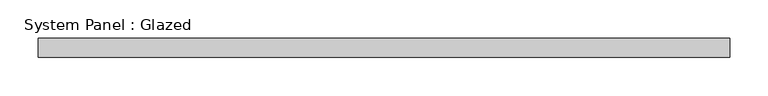
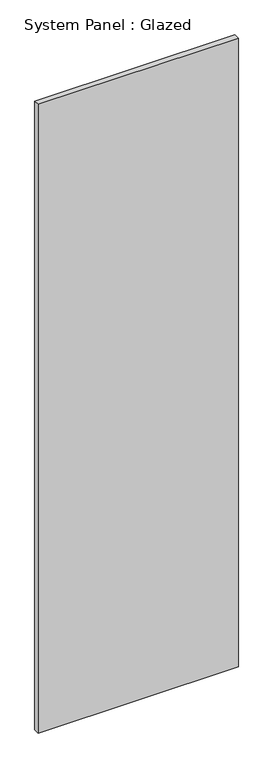
"""IFC4 building model written with IfcOpenShell, lengths in millimetres: plate geometry, System Panel : Glazed."""

from ifc_helpers import new_model, si_unit, origin, origin_with_axes, place, context, project, spatial, polyline, outline, extrude, source, transform, mapped, element, save


def system_panel_glazed_ff4fe8f0(model_context):
    return source(origin(), model_context, "Body", "SweptSolid", [
        extrude(outline(polyline([(452.482, 24.5), (-452.482, 24.5), (-452.482, 49.5), (452.482, 49.5), (452.482, 24.5)])), origin_with_axes(), (0.0, 0.0, 1.0), 3000.0),
    ])


if __name__ == "__main__":
    model = new_model("IFC4")
    model_context = context("Model", 3, world=origin())
    ifc_project = project(units=[si_unit("LENGTHUNIT", "METRE", prefix="MILLI")], contexts=[model_context])
    site = spatial("IfcSite", under=ifc_project)
    building = spatial("IfcBuilding", under=site)
    placement = place(None, origin())
    system_panel_glazed_shape = system_panel_glazed_ff4fe8f0(model_context)
    element("IfcPlate", 1, ObjectType="System Panel : Glazed", at=placement, inside=building, context=model_context, shape_type="MappedRepresentation", body=[
        mapped(system_panel_glazed_shape, transform((0.0, 0.0, 0.0), x_axis=(1.0, 0.0, 0.0), y_axis=(0.0, 1.0, 0.0), z_axis=(0.0, 0.0, 1.0))),
    ])
    save(model, "model.ifc")

# Revit data of these elements
# Type "System Panel : Glazed"
#   Keynote = "H11"
#   Construction Type Id = "GSP4R"
#   Analytic Construction = "1/8 in Pilkington single glazing"
#   Visual Light Transmittance = 0.9
#   Solar Heat Gain Coefficient = 0.86
#   Heat Transfer Coefficient (U) = 6.7069 W/(m²·K)
#   Define Thermal Properties by = 1
# Element 1 (IfcPlate, "System Panel : Glazed")
#   Materials on its faces: "Glass"
# Materials
#   "Glass": class "Glass", colour RGB 0 128 192, transparency 0.9, Description = "Soda Lime Glass", Cost = 0
